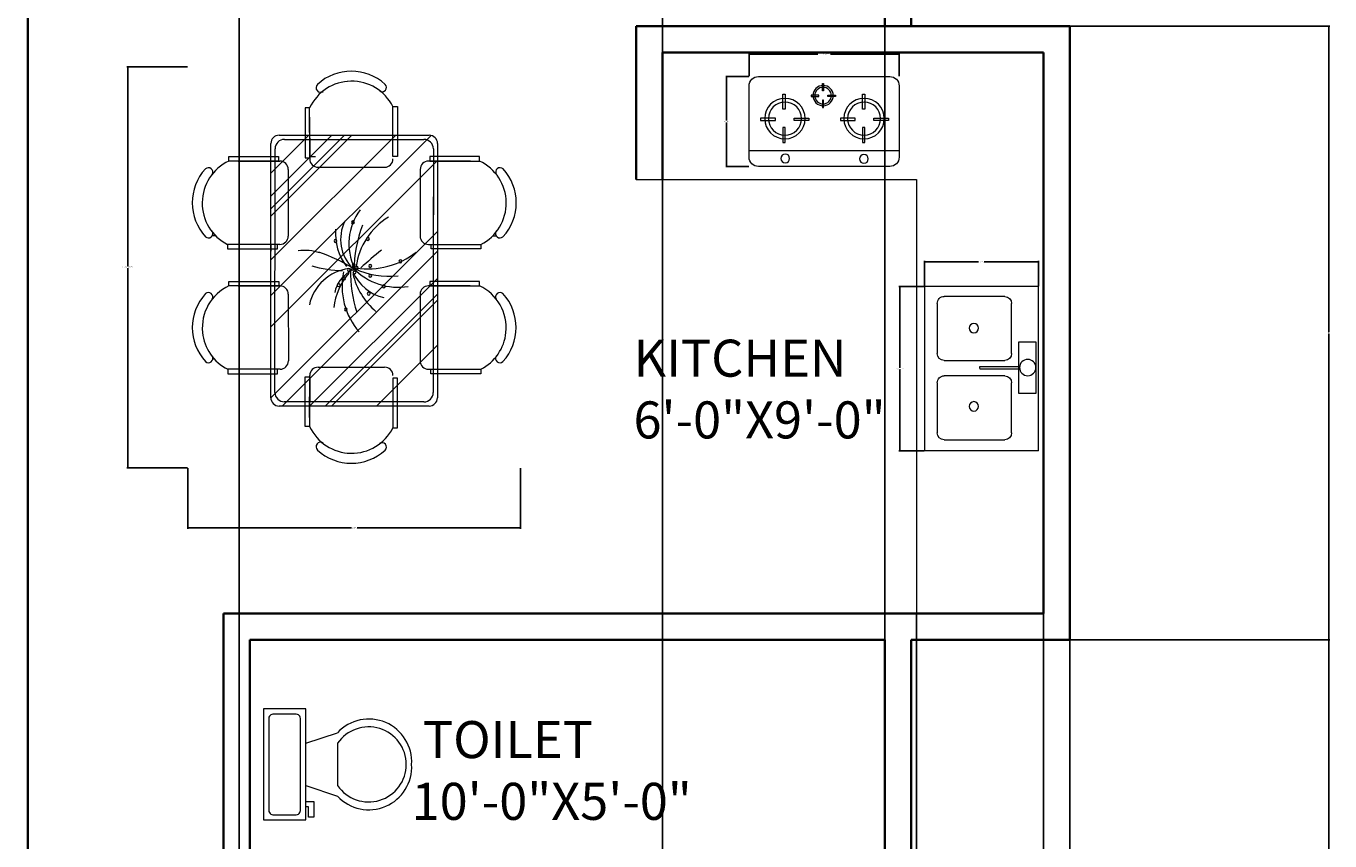
# Model space of a CAD drawing. Units: inches. Extents: x 3731 to 4318, y 1310 to 2388.
# Tile 31 of 57: x 4072 to 4318, y 1554 to 1708. Entities that reach past the tile are written whole.
import ezdxf

# ---------------------------------------------------------------- set-up
doc = ezdxf.new("R2010")
doc.units = ezdxf.units.IN
for name, color, linetype, lineweight in [('A-ANNO-DIMS', 2, 'Continuous', 18), ('A-AREA-IDEN', 7, 'Continuous', 18), ('A-EQPM', 8, 'Continuous', 18), ('A-FLOR-CASE', 8, 'Continuous', 18), ('A-FLOR-FIXT', 9, 'Continuous', 18), ('A-FURN', 8, 'Continuous', 13), ('A-WALL', 7, 'Continuous', 35)]:
    doc.layers.add(name, color=color, linetype=linetype, lineweight=lineweight)
doc.styles.get("Standard").update_dxf_attribs({"font": 'arial.ttf'})
doc.dimstyles.get("Standard").update_dxf_attribs({"dimtxt": 0.18, "dimasz": 0.18, "dimexe": 0.18, "dimexo": 0.0625, "dimgap": 0.09, "dimtad": 0, "dimtih": 1, "dimtoh": 1, "dimdec": 4, "dimzin": 0, "dimdsep": 46, "dimtxsty": 'Standard', "dimcen": 0.09, "dimadec": 0, "dimazin": 0, "dimtfac": 1, "dimtdec": 4, "dimtofl": 0, "dimtmove": 0, "dimatfit": 3, "dimfxl": 1, "dimtolj": 1, "dimtzin": 0, "dimarcsym": 0})

# ---------------------------------------------------------------- blocks, each defined once
blk = doc.blocks.new('A$C6327331B')
for p, q in [((790.8, 678.3), (790.8, 696.4)), ((790.8, 678.3), (790.8, 696.4)), ((1381.3, 692.8), (1381.3, 686.2)), ((1381.3, 692.8), (1381.3, 686.2)), ((410.1, 615.8), (410, 377)), ((410.1, 615.8), (410, 377)), ((431.6, 615.8), (410.1, 615.8)), ((431.6, 615.8), (410.1, 615.8)), ((431.4, 376.9), (431.6, 615.8)), ((431.4, 376.9), (431.6, 615.8)), ((431.5, 571.8), (431.4, 370.8)), ((431.5, 571.8), (431.4, 370.8)), ((831.4, 382.9), (831.6, 621.7)), ((831.4, 382.9), (831.6, 621.7)), ((831.4, 370.6), (831.5, 571.6)), ((831.4, 370.6), (831.5, 571.6)), ((831.6, 621.7), (853, 621.7)), ((831.6, 621.7), (853, 621.7)), ((853, 621.7), (852.9, 382.9)), ((853, 621.7), (852.9, 382.9)), ((1009.3, 615.5), (1009.2, 376.7)), ((1009.3, 615.5), (1009.2, 376.7)), ((1030.7, 615.5), (1009.3, 615.5)), ((1030.7, 615.5), (1009.3, 615.5)), ((1030.6, 376.6), (1030.7, 615.5)), ((1030.6, 376.6), (1030.7, 615.5)), ((1030.7, 571.5), (1030.6, 370.5)), ((1030.7, 571.5), (1030.6, 370.5)), ((1430.6, 382.6), (1430.7, 621.4)), ((1430.6, 382.6), (1430.7, 621.4)), ((1430.6, 370.3), (1430.7, 571.3)), ((1430.6, 370.3), (1430.7, 571.3)), ((1430.7, 621.4), (1452.2, 621.4)), ((1430.7, 621.4), (1452.2, 621.4)), ((1452.2, 621.4), (1452, 382.6)), ((1452.2, 621.4), (1452, 382.6)), ((1075.9, -386.3), (308.5, 383.1)), ((1075.9, -386.3), (308.5, 383.1)), ((347.5, 414), (831.5, 413.8)), ((347.5, 414), (831.5, 413.8)), ((372.5, 394), (831.4, 393.8)), ((372.5, 394), (1009.2, 393.7)), ((410, 377), (431.4, 376.9)), ((410, 377), (431.4, 376.9)), ((1226.3, -386.4), (428, 414)), ((1226.3, -386.4), (428, 414)), ((1567.1, -386.6), (768.8, 413.8)), ((1567.1, -386.6), (768.8, 413.8)), ((852.9, 382.9), (831.4, 382.9)), ((852.9, 382.9), (831.4, 382.9)), ((831.5, 413.8), (1567.5, 413.4)), ((1607.1, -331.3), (864.1, 413.8)), ((1607.1, -331.3), (864.1, 413.8)), ((1607.2, -200.8), (994.4, 413.7)), ((1607.2, -200.8), (994.4, 413.7)), ((1009.2, 413.7), (1567.5, 413.4)), ((1009.2, 393.7), (1542.5, 393.4)), ((1009.2, 376.7), (1030.6, 376.6)), ((1009.2, 376.7), (1030.6, 376.6)), ((1607.2, -125.5), (1069.5, 413.7)), ((1607.2, -125.5), (1069.5, 413.7)), ((1607.2, -95.4), (1099.6, 413.6)), ((1607.2, -95.4), (1099.6, 413.6)), ((1607.3, 120.5), (1315.1, 413.5)), ((1607.3, 120.5), (1315.1, 413.5)), ((1415.7, 413.4), (1415.7, 413.5)), ((1415.7, 413.4), (1415.7, 413.5)), ((1452, 382.6), (1430.6, 382.6)), ((1452, 382.6), (1430.6, 382.6)), ((307.1, -346), (307.5, 374)), ((307.1, -346), (307.5, 374)), ((327.1, -321), (327.5, 349)), ((471.4, 330.8), (791.4, 330.6)), ((471.4, 330.8), (791.4, 330.6)), ((1070.6, 330.5), (1390.6, 330.3)), ((1070.6, 330.5), (1390.6, 330.3)), ((1587.5, 348.4), (1587.1, -321.6)), ((1607.5, 373.4), (1607.1, -346.6)), ((1607.5, 373.4), (1607.1, -346.6)), ((169.9, 221.5), (408.7, 221.6)), ((169.9, 221.5), (408.7, 221.6)), ((169.9, 200.1), (169.9, 221.5)), ((169.9, 200.1), (169.9, 221.5)), ((408.7, 200.2), (169.9, 200.1)), ((408.7, 200.2), (169.9, 200.1)), ((905.5, -386.3), (307.4, 213.5)), ((905.5, -386.3), (307.4, 213.5)), ((408.7, 221.6), (408.7, 200.2)), ((408.7, 221.6), (408.7, 200.2)), ((1473.3, 221.6), (1473.3, 200.2)), ((1473.3, 221.6), (1473.3, 200.2)), ((1712.1, 221.5), (1473.3, 221.6)), ((1712.1, 221.5), (1473.3, 221.6)), ((1473.3, 200.2), (1712.1, 200.1)), ((1473.3, 200.2), (1712.1, 200.1)), ((1712.1, 200.1), (1712.1, 221.5)), ((1712.1, 200.1), (1712.1, 221.5)), ((461.2, -159.8), (461, 160.2)), ((461.2, -159.8), (461, 160.2)), ((1420.8, -159.8), (1420.9, 160.2)), ((1420.8, -159.8), (1420.9, 160.2)), ((695.1, -386.2), (307.3, 2.7)), ((695.1, -386.2), (307.3, 2.7)), ((44.6, -20.2), (44.5, -20.1)), ((44.6, -20.2), (44.5, -20.1)), ((660, -386.1), (307.3, -32.5)), ((660, -386.1), (307.3, -32.5)), ((1837.4, -20.2), (1837.5, -20.1)), ((1837.4, -20.2), (1837.5, -20.1)), ((599.8, -386.1), (307.2, -92.7)), ((599.8, -386.1), (307.2, -92.7)), ((408.7, -193.6), (408.7, -172.1)), ((408.7, -193.6), (408.7, -172.1)), ((415.1, -199.8), (176.2, -199.9)), ((415.1, -199.8), (176.2, -199.9)), ((176.2, -199.9), (176.2, -221.3)), ((176.2, -199.9), (176.2, -221.3)), ((176.2, -221.3), (415.1, -221.2)), ((176.2, -221.3), (415.1, -221.2)), ((220.2, -199.9), (421.2, -199.8)), ((220.2, -199.9), (421.2, -199.8)), ((489.6, -386), (307.2, -203.2)), ((489.6, -386), (307.2, -203.2)), ((415.1, -221.2), (415.1, -199.8)), ((415.1, -221.2), (415.1, -199.8)), ((1661.8, -199.9), (1460.8, -199.8)), ((1661.8, -199.9), (1460.8, -199.8)), ((1466.9, -221.2), (1466.9, -199.8)), ((1466.9, -221.2), (1466.9, -199.8)), ((1466.9, -199.8), (1705.7, -199.9)), ((1466.9, -199.8), (1705.7, -199.9)), ((1705.7, -221.3), (1466.9, -221.2)), ((1705.7, -221.3), (1466.9, -221.2)), ((1705.7, -199.9), (1705.7, -221.3)), ((1705.7, -199.9), (1705.7, -221.3)), ((471.4, -302.7), (791.4, -302.5)), ((471.4, -302.7), (791.4, -302.5)), ((1070.6, -302.4), (1390.6, -302.2)), ((1070.6, -302.4), (1390.6, -302.2)), ((1542.1, -366.6), (372.1, -366)), ((410.1, -587.7), (410, -348.9)), ((410.1, -587.7), (410, -348.9)), ((410, -348.9), (431.4, -348.9)), ((410, -348.9), (431.4, -348.9)), ((431.5, -543.7), (431.4, -342.7)), ((431.5, -543.7), (431.4, -342.7)), ((431.4, -348.9), (431.6, -587.7)), ((431.4, -348.9), (431.6, -587.7)), ((831.4, -342.5), (831.5, -543.5)), ((831.4, -342.5), (831.5, -543.5)), ((831.4, -354.8), (831.6, -593.6)), ((831.4, -354.8), (831.6, -593.6)), ((852.9, -354.8), (831.4, -354.8)), ((852.9, -354.8), (831.4, -354.8)), ((853, -593.6), (852.9, -354.8)), ((853, -593.6), (852.9, -354.8)), ((1009.2, -348.6), (1030.6, -348.5)), ((1009.2, -348.6), (1030.6, -348.5)), ((1009.3, -587.4), (1009.2, -348.6)), ((1009.3, -587.4), (1009.2, -348.6)), ((1030.7, -543.4), (1030.6, -342.4)), ((1030.7, -543.4), (1030.6, -342.4)), ((1030.6, -348.5), (1030.7, -587.4)), ((1030.6, -348.5), (1030.7, -587.4)), ((1430.6, -342.2), (1430.7, -543.2)), ((1430.6, -342.2), (1430.7, -543.2)), ((1430.6, -354.5), (1430.7, -593.3)), ((1430.6, -354.5), (1430.7, -593.3)), ((1452, -354.5), (1430.6, -354.5)), ((1452, -354.5), (1430.6, -354.5)), ((1452.2, -593.3), (1452, -354.5)), ((1452.2, -593.3), (1452, -354.5)), ((1567.1, -386.6), (347.1, -386)), ((1567.1, -386.6), (347.1, -386)), ((831.5, -385.7), (864.1, -385.7)), ((831.5, -385.7), (864.1, -385.7)), ((1415.7, -385.3), (1415.7, -385.4)), ((1415.7, -385.3), (1415.7, -385.4)), ((431.6, -587.7), (410.1, -587.7)), ((431.6, -587.7), (410.1, -587.7)), ((831.6, -593.6), (853, -593.6)), ((831.6, -593.6), (853, -593.6)), ((1030.7, -587.4), (1009.3, -587.4)), ((1030.7, -587.4), (1009.3, -587.4)), ((1430.7, -593.3), (1452.2, -593.3)), ((1430.7, -593.3), (1452.2, -593.3)), ((790.8, -650.2), (790.8, -668.4)), ((790.8, -650.2), (790.8, -668.4)), ((1381.3, -664.7), (1381.3, -658.1)), ((1381.3, -664.7), (1381.3, -658.1))]:
    blk.add_line(p, q)
for centre, radius, start, end in [((631.5, 550.5), 241.3, 47.46915, 132.47205), ((631.5, 550.5), 241.3, 47.46915, 132.47205), ((1230.7, 550.2), 241.3, 47.46915, 132.47205), ((1230.7, 550.2), 241.3, 47.46915, 132.47205), ((633, 521.6), 222.4, 26.76564, 154.93691), ((633, 521.6), 222.4, 26.76564, 154.93691), ((484.3, 714.2), 21.2, 137.64965, 300.34124), ((484.3, 714.2), 21.2, 137.64965, 300.34124), ((779, 714), 21.2, 239.59996, 42.29154), ((779, 714), 21.2, 239.59996, 42.29154), ((1232.2, 521.3), 222.4, 84.42654, 154.93691), ((1232.2, 521.3), 222.4, 84.42654, 154.93691), ((1083.4, 713.9), 21.2, 137.64965, 300.34124), ((1083.4, 713.9), 21.2, 137.64965, 300.34124), ((1232.2, 521.3), 222.4, 26.76564, 84.42654), ((1232.2, 521.3), 222.4, 26.76564, 84.42654), ((1378.1, 713.7), 21.2, 239.59996, 42.29154), ((1378.1, 713.7), 21.2, 239.59996, 42.29154), ((347.5, 374), 40, 89.9706, 179.9706), ((347.5, 374), 40, 89.9706, 179.9706), ((372.5, 349), 45, 89.9706, 179.9706), ((1542.5, 348.4), 45, 359.9706, 89.9706), ((1567.5, 373.4), 40, 359.9706, 89.9706), ((1567.5, 373.4), 40, 359.9706, 89.9706), ((471.4, 370.8), 40, 179.9706, 269.9706), ((471.4, 370.8), 40, 179.9706, 269.9706), ((791.4, 370.6), 40, 269.9706, 359.9706), ((791.4, 370.6), 40, 269.9706, 359.9706), ((1070.6, 370.5), 40, 179.9706, 269.9706), ((1070.6, 370.5), 40, 179.9706, 269.9706), ((1390.6, 370.3), 40, 269.9706, 359.9706), ((1390.6, 370.3), 40, 269.9706, 359.9706), ((574.1, 79.9), 374.6, 351.24958, 38.23328), ((737.8, 225), 299.2, 314.48606, 9.37622), ((270.2, 1.6), 222.4, 116.82445, 244.99571), ((270.2, 1.6), 222.4, 116.82445, 244.99571), ((421, 160.2), 40, 0.0294, 90.0294), ((421, 160.2), 40, 0.0294, 90.0294), ((912.6, 235.7), 6.91, 0, 180), ((912.6, 235.7), 6.91, 180, 0), ((586.4, 182.9), 398.1, 335.08876, 5.96372), ((1460.9, 160.2), 40, 89.9706, 179.9706), ((1460.9, 160.2), 40, 89.9706, 179.9706), ((1611.7, 1.6), 222.4, 295.00429, 63.17555), ((1611.7, 1.6), 222.4, 295.00429, 63.17555), ((241.3, 0.1), 241.3, 137.52795, 222.53085), ((77.6, 147.4), 21.2, 329.65876, 132.35035), ((77.6, 147.4), 21.2, 329.65876, 132.35035), ((983.2, 350.8), 331, 211.31505, 262.13779), ((2460.3, 1443.6), 2062.1, 219.04877, 222.6799), ((873.8, 207.8), 219.3, 294.09558, 346.29534), ((1033, 155.9), 6.91, 0, 180), ((1033, 155.9), 6.91, 180, 0), ((1804.4, 147.4), 21.2, 47.64965, 210.34124), ((1804.4, 147.4), 21.2, 47.64965, 210.34124), ((1640.7, 0.1), 241.3, 317.46915, 42.47205), ((1640.7, 0.1), 241.3, 317.46915, 42.47205), ((805, 79.9), 6.91, 0, 180), ((805, 79.9), 6.91, 180, 0), ((934.8, 91.3), 6.91, 0, 180), ((934.8, 91.3), 6.91, 180, 0), ((897.1, 334.6), 335.6, 283.04524, 319.77663), ((982.3, 91.3), 6.91, 0, 180), ((982.3, 91.3), 6.91, 180, 0), ((1067.8, 83.7), 6.91, 0, 180), ((1067.8, 83.7), 6.91, 180, 0), ((826.9, 258.5), 270.1, 233.32313, 295.76326), ((725.8, 7.7), 6.91, 0, 180), ((725.8, 7.7), 6.91, 180, 0), ((807.8, 143), 194.5, 242.99086, 315.91017), ((985.1, 750.7), 739.8, 250.5249, 267.82437), ((1747.6, -469.5), 933.6, 148.98728, 160.36101), ((931.7, 11.5), 6.91, 0, 180), ((931.7, 11.5), 6.91, 180, 0), ((944.3, 26.7), 6.91, 0, 180), ((944.3, 26.7), 6.91, 180, 0), ((947.5, 3.9), 6.91, 0, 180), ((947.5, 3.9), 6.91, 180, 0), ((970.7, 574.8), 578.8, 268.32856, 288.729), ((966.5, 15.3), 6.91, 0, 180), ((966.5, 15.3), 6.91, 180, 0), ((1030.3, 292.7), 337.4, 258.55155, 310.98153), ((776.7, 191.6), 268.2, 265.87406, 306.95584), ((392.7, -33), 564.4, 343.85612, 359.11051), ((953.8, -11.3), 6.91, 0, 180), ((953.8, -11.3), 6.91, 180, 0), ((1167.7, 15.7), 221.9, 186.99045, 258.02836), ((1090.6, 62.7), 145.4, 208.89012, 258.45792), ((1166.2, 212.9), 298.2, 228.7581, 263.8624), ((995, -34.1), 6.91, 0, 180), ((995, -34.1), 6.91, 180, 0), ((1026.7, -60.7), 6.91, 0, 180), ((1026.7, -60.7), 6.91, 180, 0), ((1143.8, -26.5), 6.91, 0, 180), ((1143.8, -26.5), 6.91, 180, 0), ((814.5, -75.9), 6.91, 0, 180), ((814.5, -75.9), 6.91, 180, 0), ((79, -146.7), 22.5, 226.37763, 29.88821), ((79, -146.7), 22.5, 226.37763, 29.88821), ((421.2, -159.8), 40, 270.0294, 0.0294), ((421.2, -159.8), 40, 270.0294, 0.0294), ((1112.9, -226), 252.6, 162.94564, 186.48138), ((1460.8, -159.8), 40, 179.9706, 269.9706), ((1460.8, -159.8), 40, 179.9706, 269.9706), ((1803, -146.7), 22.5, 150.11179, 313.62237), ((1803, -146.7), 22.5, 150.11179, 313.62237), ((471.4, -342.7), 40, 90.0294, 180.0294), ((471.4, -342.7), 40, 90.0294, 180.0294), ((791.4, -342.5), 40, 0.0294, 90.0294), ((791.4, -342.5), 40, 0.0294, 90.0294), ((1070.6, -342.4), 40, 90.0294, 180.0294), ((1070.6, -342.4), 40, 90.0294, 180.0294), ((1390.6, -342.2), 40, 0.0294, 90.0294), ((1390.6, -342.2), 40, 0.0294, 90.0294), ((347.1, -346), 40, 179.9706, 269.9706), ((347.1, -346), 40, 179.9706, 269.9706), ((372.1, -321), 45, 179.9706, 269.9706), ((1542.1, -321.6), 45, 269.9706, 359.9706), ((1567.1, -346.6), 40, 269.9706, 359.9706), ((1567.1, -346.6), 40, 269.9706, 359.9706), ((633, -493.5), 222.4, 205.06309, 333.23436), ((633, -493.5), 222.4, 205.06309, 333.23436), ((1232.2, -493.2), 222.4, 205.06309, 275.57346), ((1232.2, -493.2), 222.4, 205.06309, 275.57346), ((1232.2, -493.2), 222.4, 275.57346, 333.23436), ((1232.2, -493.2), 222.4, 275.57346, 333.23436), ((484.3, -686.1), 21.2, 59.65876, 222.35035), ((484.3, -686.1), 21.2, 59.65876, 222.35035), ((779, -686), 21.2, 317.70846, 120.40004), ((779, -686), 21.2, 317.70846, 120.40004), ((1083.4, -685.8), 21.2, 59.65876, 222.35035), ((1083.4, -685.8), 21.2, 59.65876, 222.35035), ((1378.1, -685.6), 21.2, 317.70846, 120.40004), ((1378.1, -685.6), 21.2, 317.70846, 120.40004), ((631.5, -522.4), 241.3, 227.52795, 312.53085), ((631.5, -522.4), 241.3, 227.52795, 312.53085), ((1230.7, -522.1), 241.3, 227.52795, 312.53085), ((1230.7, -522.1), 241.3, 227.52795, 312.53085)]:
    blk.add_arc(centre, radius, start, end)
at = {"width": 0.8, "flags": 9}
for tag in ['XSIZE', 'YSIZE']:
    blk.add_attdef(tag, (945.2, 11.4), '', height=0.23, rotation=180, dxfattribs=at)
blk = doc.blocks.new('*U14')
for p, q in [((9.5, -6), (9.5, -2)), ((-10, -8.5), (-8, -8.5)), ((-10, -9.5), (-10, -8.5)), ((-7, -9.5), (-10, -9.5)), ((-8, -8.5), (-8, -8)), ((-7, -8), (-7, -9.5)), ((-4, -8), (-6, -14)), ((4, -8), (6, -14)), ((4, -14), (-4, -14))]:
    blk.add_line(p, q)
blk.add_lwpolyline([(10.5, -8), (10.5, 0), (-10.5, 0), (-10.5, -8)], close=True)
for points in [[(-9.5, -2), (-9.5, -6)], [(8.5, -1), (-8.5, -1)], [(-8.5, -7), (8.5, -7)]]:
    blk.add_lwpolyline(points)
for centre, radius, start, end in [((-8.625, -1.875), 0.8839, 81.8699, 188.1301), ((8.625, -1.875), 0.8839, 351.8699, 98.1301), ((-8.625, -6.125), 0.8839, 171.869898, 278.1301), ((8.625, -6.125), 0.8839, 261.8699, 8.1301), ((-0.4772, -19.9188), 8.0953, 133.01722, 273.38), ((0.0374, -19.8731), 7.127, 124.50543, 269.7), ((-0.0373, -19.8731), 7.127, 270.3, 55.4946), ((0.4773, -19.9188), 8.0953, 266.62, 46.9828)]:
    blk.add_arc(centre, radius, start, end)
blk = doc.blocks.new('A$C2A3C6842')
for p, q in [((0, 45), (0, 387)), ((45, 432), (675, 432)), ((351.6, 363.3), (351.6, 398.9)), ((351.6, 398.9), (357.3, 398.9)), ((357.3, 398.9), (357.3, 363.3)), ((720, 387), (720, 45)), ((161.8, 346.9), (173.2, 346.9)), ((161.8, 275.6), (161.8, 346.9)), ((173.2, 346.9), (173.2, 275.6)), ((298.4, 341.9), (298.4, 336.2)), ((334, 341.9), (298.4, 341.9)), ((298.4, 336.2), (334, 336.2)), ((334, 336.2), (334, 341.9)), ((357.3, 363.3), (351.6, 363.3)), ((357.3, 318.8), (351.6, 318.8)), ((351.6, 318.8), (351.6, 283.1)), ((357.3, 283.1), (357.3, 318.8)), ((378.5, 336.2), (378.5, 341.9)), ((378.5, 341.9), (414.2, 341.9)), ((414.2, 336.2), (378.5, 336.2)), ((414.2, 341.9), (414.2, 336.2)), ((544.7, 346.9), (556.1, 346.9)), ((544.7, 275.6), (544.7, 346.9)), ((556.1, 346.9), (556.1, 275.6)), ((173.2, 275.6), (161.8, 275.6)), ((351.6, 283.1), (357.3, 283.1)), ((556.1, 275.6), (544.7, 275.6)), ((55.3, 232.9), (55.3, 221.5)), ((126.6, 232.9), (55.3, 232.9)), ((55.3, 221.5), (126.6, 221.5)), ((126.6, 221.5), (126.6, 232.9)), ((215.6, 221.5), (215.6, 232.9)), ((215.6, 232.9), (286.9, 232.9)), ((286.9, 221.5), (215.6, 221.5)), ((286.9, 232.9), (286.9, 221.5)), ((438.2, 232.9), (438.2, 221.5)), ((509.5, 232.9), (438.2, 232.9)), ((438.2, 221.5), (509.5, 221.5)), ((509.5, 221.5), (509.5, 232.9)), ((598.5, 232.9), (669.8, 232.9)), ((598.5, 221.5), (598.5, 232.9)), ((669.8, 221.5), (598.5, 221.5)), ((669.8, 232.9), (669.8, 221.5)), ((173.2, 186.6), (161.8, 186.6)), ((161.8, 186.6), (161.8, 115.3)), ((173.2, 115.3), (173.2, 186.6)), ((556.1, 186.6), (544.7, 186.6)), ((544.7, 186.6), (544.7, 115.3)), ((556.1, 115.3), (556.1, 186.6)), ((1.2, 76.7), (719.9, 76.7)), ((161.8, 115.3), (173.2, 115.3)), ((544.7, 115.3), (556.1, 115.3)), ((675, 0), (45, 0))]:
    blk.add_line(p, q)
at = {"extrusion": (0, -1e-16, -1)}
for centre, major_axis, start_param, end_param in [((45, 387), (31.8, 31.8), 3.926991, 5.497787), ((172.2, 229.8), (-97.3, 0.1), -0.001099, 6.282086), ((551.8, 229.8), (-97.3, 0.1), -0.001099, 6.282086), ((173.7, 39), (-14.8, 14.8), 5.497787, 11.780972)]:
    blk.add_ellipse(centre, major_axis=major_axis, ratio=1, start_param=start_param, end_param=end_param, dxfattribs=at)
at = {"extrusion": (-1e-16, -1e-16, -1)}
blk.add_ellipse((355.1, 340.4), major_axis=(48.7, 0.1), ratio=1, start_param=3.144125, end_param=9.42731, dxfattribs=at)
at = {"extrusion": (-1e-16, 0, -1)}
for centre, major_axis, start_param, end_param in [((355.1, 340.4), (-39.7, 0), -0.000334, 6.282851), ((45, 45), (-31.8, 31.8), 3.926991, 5.497787)]:
    blk.add_ellipse(centre, major_axis=major_axis, ratio=1, start_param=start_param, end_param=end_param, dxfattribs=at)
at = {"extrusion": (0, 1e-16, -1)}
blk.add_ellipse((675, 387), major_axis=(-31.8, 31.8), ratio=1, start_param=0.785398, end_param=2.356194, dxfattribs=at)
at = {"extrusion": (-1e-16, -4e-16, -1)}
for centre in [(172.2, 229.8), (551.8, 229.8)]:
    blk.add_ellipse(centre, major_axis=(-79.3, 0), ratio=1, start_param=-0.0002116186602152, end_param=6.282973688519371, dxfattribs=at)
at = {"extrusion": (2e-16, -2e-16, -1)}
blk.add_ellipse((551.4, 36.4), major_axis=(14.8, 14.8), ratio=1, start_param=3.926991, end_param=10.210176, dxfattribs=at)
at = {"extrusion": (-2e-16, 1e-16, -1)}
blk.add_ellipse((675, 45), major_axis=(31.8, 31.8), ratio=1, start_param=0.785398, end_param=2.356194, dxfattribs=at)
at = {"text_generation_flag": 4, "flags": 9}
for tag in ['XSIZE', 'YSIZE']:
    blk.add_attdef(tag, (361.3, 264.9), '', height=0.45, rotation=180, dxfattribs=at)
blk = doc.blocks.new('A$C3AD04490')
for p, q in [((0, 640.7), (0, 0)), ((0, 640.7), (924.9, 640.7)), ((614, 627.3), (322.5, 627.3)), ((322.5, 627.3), (322.5, 531.5)), ((614, 531.5), (614, 627.3)), ((924.9, 640.7), (924.9, 0)), ((322.5, 531.5), (614, 531.5)), ((462.6, 311.9), (462.6, 537.2)), ((473.8, 536.8), (473.8, 311.9)), ((62.3, 110.9), (62.3, 451.4)), ((101.4, 490.5), (383.1, 490.5)), ((422.3, 451.4), (422.3, 110.9)), ((508.8, 110.9), (508.8, 451.4)), ((547.9, 490.5), (829.6, 490.5)), ((868.8, 451.4), (868.8, 110.9)), ((463.4, 310.9), (474.3, 310.9)), ((383.1, 71.7), (101.4, 71.7)), ((829.6, 71.7), (547.9, 71.7)), ((924.9, 0), (0, 0))]:
    blk.add_line(p, q)
for centre, radius in [((469, 581.2), 45.9), ((250.7, 278.1), 26.4), ((690.5, 278.1), 26.4)]:
    blk.add_circle(centre, radius)
for centre, start, end in [((101.4, 451.4), 90, 180), ((383.1, 451.4), 0, 90), ((547.9, 451.4), 90, 180), ((829.6, 451.4), 0, 90), ((101.4, 110.9), 180, 270), ((383.1, 110.9), 270, 0), ((547.9, 110.9), 180, 270), ((829.6, 110.9), 270, 0)]:
    blk.add_arc(centre, 39.1, start, end)
blk = doc.blocks.new('*D24')
at = {"layer": 'A-ANNO-DIMS', "color": 0, "lineweight": -2, "transparency": 16777216}
for p, q in [((4102.42, 1700.68), (4090.94, 1700.68)), ((4091.12, 1700.5), (4091.12, 1662.99)), ((4091.12, 1625.1), (4091.12, 1662.62)), ((4102.42, 1624.92), (4090.94, 1624.92))]:
    blk.add_line(p, q, dxfattribs=at)
at = {"layer": 'A-ANNO-DIMS', "color": 0, "transparency": 16777216}
for points in [[(4091.09, 1700.5), (4091.15, 1700.5), (4091.12, 1700.68)], [(4091.09, 1625.1), (4091.15, 1625.1), (4091.12, 1624.92)]]:
    blk.add_solid(points, dxfattribs=at)
at = {"layer": 'Defpoints', "color": 0, "transparency": 16777216}
for p in [(4102.48, 1700.68), (4091.12, 1624.92), (4102.48, 1624.92)]:
    blk.add_point(p, dxfattribs=at)
at = {"layer": 'A-ANNO-DIMS', "color": 0, "transparency": 16777216, "insert": (4091.12, 1662.8), "char_height": 0.18, "attachment_point": 5}
blk.add_mtext('\\A1;DINING SET 76 TYP.', dxfattribs=at)
blk = doc.blocks.new('*D25')
at = {"layer": 'A-ANNO-DIMS', "color": 0, "lineweight": -2, "transparency": 16777216}
for p, q in [((4102.48, 1624.86), (4102.48, 1613.38)), ((4165.39, 1624.86), (4165.39, 1613.38)), ((4102.66, 1613.56), (4133.41, 1613.56)), ((4165.21, 1613.56), (4134.46, 1613.56))]:
    blk.add_line(p, q, dxfattribs=at)
at = {"layer": 'A-ANNO-DIMS', "color": 0, "transparency": 16777216}
for points in [[(4102.66, 1613.59), (4102.66, 1613.53), (4102.48, 1613.56)], [(4165.21, 1613.59), (4165.21, 1613.53), (4165.39, 1613.56)]]:
    blk.add_solid(points, dxfattribs=at)
at = {"layer": 'Defpoints', "color": 0, "transparency": 16777216}
for p in [(4102.48, 1624.92), (4165.39, 1624.92), (4165.39, 1613.56)]:
    blk.add_point(p, dxfattribs=at)
at = {"layer": 'A-ANNO-DIMS', "color": 0, "transparency": 16777216, "insert": (4133.93, 1613.56), "char_height": 0.18, "attachment_point": 5}
blk.add_mtext('\\A1;63 TYP.', dxfattribs=at)
blk = doc.blocks.new('*D26')
at = {"layer": 'A-ANNO-DIMS', "color": 0, "lineweight": -2, "transparency": 16777216}
for p, q in [((4241.66, 1659.17), (4236.88, 1659.17)), ((4237.06, 1658.99), (4237.06, 1643.82)), ((4237.06, 1628.27), (4237.06, 1643.45)), ((4241.66, 1628.09), (4236.88, 1628.09))]:
    blk.add_line(p, q, dxfattribs=at)
at = {"layer": 'A-ANNO-DIMS', "color": 0, "transparency": 16777216}
for points in [[(4237.03, 1658.99), (4237.09, 1658.99), (4237.06, 1659.17)], [(4237.03, 1628.27), (4237.09, 1628.27), (4237.06, 1628.09)]]:
    blk.add_solid(points, dxfattribs=at)
at = {"layer": 'Defpoints', "color": 0, "transparency": 16777216}
for p in [(4237.06, 1659.17), (4241.72, 1659.17), (4241.72, 1628.09)]:
    blk.add_point(p, dxfattribs=at)
at = {"layer": 'A-ANNO-DIMS', "color": 0, "transparency": 16777216, "insert": (4237.06, 1643.63), "char_height": 0.18, "attachment_point": 5}
blk.add_mtext('\\A1;SINK 31 TYP.', dxfattribs=at)
blk = doc.blocks.new('*D27')
at = {"layer": 'A-ANNO-DIMS', "color": 0, "lineweight": -2, "transparency": 16777216}
for p, q in [((4241.72, 1659.23), (4241.72, 1664.01)), ((4241.9, 1663.83), (4251.96, 1663.83)), ((4263.07, 1663.83), (4253.02, 1663.83)), ((4263.25, 1659.23), (4263.25, 1664.01))]:
    blk.add_line(p, q, dxfattribs=at)
at = {"layer": 'A-ANNO-DIMS', "color": 0, "transparency": 16777216}
for points in [[(4241.9, 1663.86), (4241.9, 1663.8), (4241.72, 1663.83)], [(4263.07, 1663.86), (4263.07, 1663.8), (4263.25, 1663.83)]]:
    blk.add_solid(points, dxfattribs=at)
at = {"layer": 'Defpoints', "color": 0, "transparency": 16777216}
for p in [(4263.25, 1663.83), (4241.72, 1659.17), (4263.25, 1659.17)]:
    blk.add_point(p, dxfattribs=at)
at = {"layer": 'A-ANNO-DIMS', "color": 0, "transparency": 16777216, "insert": (4252.49, 1663.83), "char_height": 0.18, "attachment_point": 5}
blk.add_mtext('\\A1;22 TYP.', dxfattribs=at)
blk = doc.blocks.new('*D28')
at = {"layer": 'A-ANNO-DIMS', "color": 0, "lineweight": -2, "transparency": 16777216}
for p, q in [((4208.58, 1698.91), (4208.58, 1703.28)), ((4208.76, 1703.1), (4221.57, 1703.1)), ((4236.75, 1703.1), (4223.95, 1703.1)), ((4236.93, 1698.91), (4236.93, 1703.28))]:
    blk.add_line(p, q, dxfattribs=at)
at = {"layer": 'A-ANNO-DIMS', "color": 0, "transparency": 16777216}
for points in [[(4208.76, 1703.13), (4208.76, 1703.07), (4208.58, 1703.1)], [(4236.75, 1703.13), (4236.75, 1703.07), (4236.93, 1703.1)]]:
    blk.add_solid(points, dxfattribs=at)
at = {"layer": 'Defpoints', "color": 0, "transparency": 16777216}
for p in [(4236.93, 1703.1), (4208.58, 1698.85), (4236.93, 1698.85)]:
    blk.add_point(p, dxfattribs=at)
at = {"layer": 'A-ANNO-DIMS', "color": 0, "transparency": 16777216, "insert": (4222.76, 1703.1), "char_height": 0.18, "attachment_point": 5}
blk.add_mtext('\\A1;COOKTOP 28 TYP.', dxfattribs=at)
blk = doc.blocks.new('*D29')
at = {"layer": 'A-ANNO-DIMS', "color": 0, "lineweight": -2, "transparency": 16777216}
for p, q in [((4208.52, 1698.85), (4204.15, 1698.85)), ((4204.33, 1698.67), (4204.33, 1690.53)), ((4204.33, 1682.02), (4204.33, 1690.17)), ((4208.52, 1681.84), (4204.15, 1681.84))]:
    blk.add_line(p, q, dxfattribs=at)
at = {"layer": 'A-ANNO-DIMS', "color": 0, "transparency": 16777216}
for points in [[(4204.3, 1698.67), (4204.36, 1698.67), (4204.33, 1698.85)], [(4204.3, 1682.02), (4204.36, 1682.02), (4204.33, 1681.84)]]:
    blk.add_solid(points, dxfattribs=at)
at = {"layer": 'Defpoints', "color": 0, "transparency": 16777216}
for p in [(4204.33, 1698.85), (4208.58, 1698.85), (4208.58, 1681.84)]:
    blk.add_point(p, dxfattribs=at)
at = {"layer": 'A-ANNO-DIMS', "color": 0, "transparency": 16777216, "insert": (4204.33, 1690.35), "char_height": 0.18, "attachment_point": 5}
blk.add_mtext('\\A1;17 TYP.', dxfattribs=at)
blk = doc.blocks.new('*D32')
at = {"layer": 'A-ANNO-DIMS', "color": 0, "lineweight": -2, "transparency": 16777216}
for p, q in [((4269.21, 1592.32), (4269.21, 1310.25)), ((3835.21, 1359.32), (3835.21, 1310.25)), ((3835.39, 1310.43), (4051.92, 1310.43)), ((4269.03, 1310.43), (4052.5, 1310.43))]:
    blk.add_line(p, q, dxfattribs=at)
at = {"layer": 'A-ANNO-DIMS', "color": 0, "transparency": 16777216}
for points in [[(3835.39, 1310.46), (3835.39, 1310.4), (3835.21, 1310.43)], [(4269.03, 1310.46), (4269.03, 1310.4), (4269.21, 1310.43)]]:
    blk.add_solid(points, dxfattribs=at)
at = {"layer": 'Defpoints', "color": 0, "transparency": 16777216}
for p in [(4269.21, 1592.38), (3835.21, 1359.38), (4269.21, 1310.43)]:
    blk.add_point(p, dxfattribs=at)
at = {"layer": 'A-ANNO-DIMS', "color": 0, "transparency": 16777216, "insert": (4052.21, 1310.43), "char_height": 0.18, "attachment_point": 5}
blk.add_mtext('\\A1;434', dxfattribs=at)
blk = doc.blocks.new('*D41')
at = {"layer": 'A-ANNO-DIMS', "color": 0, "lineweight": -2, "transparency": 16777216}
for p, q in [((4269.27, 1708.38), (4318.34, 1708.38)), ((4318.16, 1708.2), (4318.16, 1650.56)), ((4318.16, 1592.56), (4318.16, 1650.2)), ((4269.27, 1592.38), (4318.34, 1592.38))]:
    blk.add_line(p, q, dxfattribs=at)
at = {"layer": 'A-ANNO-DIMS', "color": 0, "transparency": 16777216}
for points in [[(4318.13, 1708.2), (4318.19, 1708.2), (4318.16, 1708.38)], [(4318.13, 1592.56), (4318.19, 1592.56), (4318.16, 1592.38)]]:
    blk.add_solid(points, dxfattribs=at)
at = {"layer": 'Defpoints', "color": 0, "transparency": 16777216}
for p in [(4269.21, 1708.38), (4318.16, 1708.38), (4269.21, 1592.38)]:
    blk.add_point(p, dxfattribs=at)
at = {"layer": 'A-ANNO-DIMS', "color": 0, "transparency": 16777216, "insert": (4318.16, 1650.38), "char_height": 0.18, "attachment_point": 5}
blk.add_mtext('\\A1;116', dxfattribs=at)
blk = doc.blocks.new('*D42')
at = {"layer": 'A-ANNO-DIMS', "color": 0, "lineweight": -2, "transparency": 16777216}
for p, q in [((4269.27, 1592.38), (4318.34, 1592.38)), ((4318.16, 1592.2), (4318.16, 1476.06)), ((4318.16, 1359.56), (4318.16, 1475.7)), ((4239.27, 1359.38), (4318.34, 1359.38))]:
    blk.add_line(p, q, dxfattribs=at)
at = {"layer": 'A-ANNO-DIMS', "color": 0, "transparency": 16777216}
for points in [[(4318.13, 1592.2), (4318.19, 1592.2), (4318.16, 1592.38)], [(4318.13, 1359.56), (4318.19, 1359.56), (4318.16, 1359.38)]]:
    blk.add_solid(points, dxfattribs=at)
at = {"layer": 'Defpoints', "color": 0, "transparency": 16777216}
for p in [(4269.21, 1592.38), (4318.16, 1592.38), (4239.21, 1359.38)]:
    blk.add_point(p, dxfattribs=at)
at = {"layer": 'A-ANNO-DIMS', "color": 0, "transparency": 16777216, "insert": (4318.16, 1475.88), "char_height": 0.18, "attachment_point": 5}
blk.add_mtext('\\A1;233', dxfattribs=at)
blk = doc.blocks.new('*D43')
at = {"layer": 'A-ANNO-DIMS', "color": 0, "lineweight": -2, "transparency": 16777216}
for p, q in [((4240.21, 1597.39), (4240.21, 1310.25)), ((4264.21, 1597.32), (4264.21, 1310.25)), ((4240.39, 1310.43), (4251.99, 1310.43)), ((4264.03, 1310.43), (4252.43, 1310.43))]:
    blk.add_line(p, q, dxfattribs=at)
at = {"layer": 'A-ANNO-DIMS', "color": 0, "transparency": 16777216}
for points in [[(4240.39, 1310.46), (4240.39, 1310.4), (4240.21, 1310.43)], [(4264.03, 1310.46), (4264.03, 1310.4), (4264.21, 1310.43)]]:
    blk.add_solid(points, dxfattribs=at)
at = {"layer": 'Defpoints', "color": 0, "transparency": 16777216}
for p in [(4240.21, 1597.45), (4264.21, 1597.38), (4264.21, 1310.43)]:
    blk.add_point(p, dxfattribs=at)
at = {"layer": 'A-ANNO-DIMS', "color": 0, "transparency": 16777216, "insert": (4252.21, 1310.43), "char_height": 0.18, "attachment_point": 5}
blk.add_mtext('\\A1;24', dxfattribs=at)
blk = doc.blocks.new('*D46')
at = {"layer": 'A-ANNO-DIMS', "color": 0, "lineweight": -2, "transparency": 16777216}
for p, q in [((4112.21, 1854.32), (4112.21, 1310.25)), ((4192.21, 1854.32), (4192.21, 1310.25)), ((4112.39, 1310.43), (4151.99, 1310.43)), ((4192.03, 1310.43), (4152.43, 1310.43))]:
    blk.add_line(p, q, dxfattribs=at)
at = {"layer": 'A-ANNO-DIMS', "color": 0, "transparency": 16777216}
for points in [[(4112.39, 1310.46), (4112.39, 1310.4), (4112.21, 1310.43)], [(4192.03, 1310.46), (4192.03, 1310.4), (4192.21, 1310.43)]]:
    blk.add_solid(points, dxfattribs=at)
at = {"layer": 'Defpoints', "color": 0, "transparency": 16777216}
for p in [(4112.21, 1854.38), (4192.21, 1854.38), (4192.21, 1310.43)]:
    blk.add_point(p, dxfattribs=at)
at = {"layer": 'A-ANNO-DIMS', "color": 0, "transparency": 16777216, "insert": (4152.21, 1310.43), "char_height": 0.18, "attachment_point": 5}
blk.add_mtext('\\A1;80', dxfattribs=at)
blk = doc.blocks.new('*D47')
at = {"layer": 'A-ANNO-DIMS', "color": 0, "lineweight": -2, "transparency": 16777216}
for p, q in [((4192.21, 1854.32), (4192.21, 1310.25)), ((4234.21, 1854.32), (4234.21, 1310.25)), ((4192.39, 1310.43), (4212.99, 1310.43)), ((4234.03, 1310.43), (4213.43, 1310.43))]:
    blk.add_line(p, q, dxfattribs=at)
at = {"layer": 'A-ANNO-DIMS', "color": 0, "transparency": 16777216}
for points in [[(4192.39, 1310.46), (4192.39, 1310.4), (4192.21, 1310.43)], [(4234.03, 1310.46), (4234.03, 1310.4), (4234.21, 1310.43)]]:
    blk.add_solid(points, dxfattribs=at)
at = {"layer": 'Defpoints', "color": 0, "transparency": 16777216}
for p in [(4192.21, 1854.38), (4234.21, 1854.38), (4234.21, 1310.43)]:
    blk.add_point(p, dxfattribs=at)
at = {"layer": 'A-ANNO-DIMS', "color": 0, "transparency": 16777216, "insert": (4213.21, 1310.43), "char_height": 0.18, "attachment_point": 5}
blk.add_mtext('\\A1;42', dxfattribs=at)

msp = doc.modelspace()

# ---------------------------------------------------------------- linework, layer by layer
at = {"layer": 'A-FLOR-CASE'}
for p, q in [((4187.21, 1679.38), (4240.21, 1679.38)), ((4240.21, 1679.38), (4240.21, 1597.45))]:
    msp.add_line(p, q, dxfattribs=at)
at = {"layer": 'A-WALL'}
for p, q in [((4239.21, 2338.38), (4239.21, 1708.38)), ((4234.21, 1849.38), (4234.21, 1708.38)), ((4072.21, 1803.38), (4072.21, 1484.38)), ((4187.21, 1708.38), (4269.21, 1708.38)), ((4187.21, 1708.38), (4187.21, 1679.38)), ((4269.21, 1708.38), (4269.21, 1592.38)), ((4192.21, 1703.38), (4264.21, 1703.38)), ((4192.21, 1703.38), (4192.21, 1679.38)), ((4264.21, 1703.38), (4264.21, 1597.38)), ((4109.21, 1597.38), (4264.21, 1597.38)), ((4109.21, 1597.38), (4109.21, 1532.38)), ((4114.21, 1592.38), (4114.21, 1532.38)), ((4114.21, 1592.38), (4234.21, 1592.38)), ((4234.21, 1592.38), (4234.21, 1532.38)), ((4239.21, 1592.38), (4239.21, 1359.38)), ((4239.21, 1592.38), (4269.21, 1592.38))]:
    msp.add_line(p, q, dxfattribs=at)

# ---------------------------------------------------------------- block references
at = {"layer": 'A-EQPM', "xscale": 0.0393700787401575, "yscale": 0.0393700787401575, "zscale": 0.0393700787401575}
msp.add_blockref('A$C2A3C6842', (4208.58, 1681.84), dxfattribs=at)
at = {"layer": 'A-FLOR-FIXT', "xscale": -0.0336022830821591, "yscale": 0.0336022830821591, "zscale": 0.0336022830821591, "rotation": 270}
msp.add_blockref('A$C3AD04490', (4241.72, 1628.09), dxfattribs=at)
at = {"layer": 'A-FLOR-FIXT', "rotation": 90}
msp.add_blockref('*U14', (4116.78, 1568.84), dxfattribs=at)
at = {"layer": 'A-FURN', "xscale": 0.0393700787401575, "yscale": 0.0393700787401575, "zscale": 0.0393700787401575, "rotation": 270}
msp.add_blockref('A$C6327331B', (4133.38, 1699.85), dxfattribs=at)

# ---------------------------------------------------------------- texts
at = {"layer": 'A-AREA-IDEN', "char_height": 7, "attachment_point": 1}
for s, width, insert in [('KITCHEN\\P6\'-0"X9\'-0"', 47.0437, (4186.72, 1649.12)), (' TOILET\\P10\'-0"X5\'-0"', 39.1687, (4144.78, 1577.03))]:
    msp.add_mtext_dynamic_manual_height_columns(s, width=width, gutter_width=12.5, heights=[0], dxfattribs=dict(at, insert=insert))

# ---------------------------------------------------------------- dimensions: what is measured, and where the dimension line sits
at = {"layer": 'A-ANNO-DIMS'}
for base, p1, p2, picture, middle in [((4192.21, 1310.43), (4112.21, 1854.38), (4192.21, 1854.38), '*D46', (4152.21, 1310.43)), ((4234.21, 1310.43), (4192.21, 1854.38), (4234.21, 1854.38), '*D47', (4213.21, 1310.43)), ((4264.21, 1310.43), (4240.21, 1597.45), (4264.21, 1597.38), '*D43', (4252.21, 1310.43)), ((4269.21, 1310.43), (3835.21, 1359.38), (4269.21, 1592.38), '*D32', (4052.21, 1310.43))]:
    dim = msp.add_linear_dim(base=base, p1=p1, p2=p2, dimstyle='Standard', override={"dimdec": 0, "dimlfac": 1, "dimrnd": 0, "dimzin": 0, "dimdsep": 46, "dimlunit": 2}, dxfattribs=at)
    dim.commit()
    dim.dimension.update_dxf_attribs({"geometry": picture, "text_midpoint": middle})
for base, p1, p2, picture, middle in [((4318.16, 1708.38), (4269.21, 1592.38), (4269.21, 1708.38), '*D41', (4318.16, 1650.38)), ((4318.16, 1592.38), (4239.21, 1359.38), (4269.21, 1592.38), '*D42', (4318.16, 1475.88))]:
    dim = msp.add_linear_dim(base=base, p1=p1, p2=p2, angle=90, dimstyle='Standard', override={"dimdec": 0, "dimlfac": 1, "dimrnd": 0, "dimzin": 0, "dimdsep": 46, "dimlunit": 2}, dxfattribs=at)
    dim.commit()
    dim.dimension.update_dxf_attribs({"geometry": picture, "text_midpoint": middle})
for base, p1, p2, text, picture, middle in [((4236.93, 1703.1), (4208.58, 1698.85), (4236.93, 1698.85), 'COOKTOP <> TYP.', '*D28', (4222.76, 1703.1)), ((4263.25, 1663.83), (4241.72, 1659.17), (4263.25, 1659.17), '<> TYP.', '*D27', (4252.49, 1663.83)), ((4165.39, 1613.56), (4102.48, 1624.92), (4165.39, 1624.92), '<> TYP.', '*D25', (4133.93, 1613.56))]:
    dim = msp.add_linear_dim(base=base, p1=p1, p2=p2, text=text, dimstyle='Standard', override={"dimdec": 0, "dimlfac": 1, "dimrnd": 0, "dimzin": 0, "dimdsep": 46, "dimlunit": 2}, dxfattribs=at)
    dim.commit()
    dim.dimension.update_dxf_attribs({"geometry": picture, "text_midpoint": middle})
for base, p1, p2, angle, text, picture, middle in [((4091.12, 1624.92), (4102.48, 1700.68), (4102.48, 1624.92), 270, 'DINING SET <> TYP.', '*D24', (4091.12, 1662.8)), ((4204.33, 1698.85), (4208.58, 1681.84), (4208.58, 1698.85), 90, '<> TYP.', '*D29', (4204.33, 1690.35)), ((4237.06, 1659.17), (4241.72, 1628.09), (4241.72, 1659.17), 90, 'SINK <> TYP.', '*D26', (4237.06, 1643.63))]:
    dim = msp.add_linear_dim(base=base, p1=p1, p2=p2, angle=angle, text=text, dimstyle='Standard', override={"dimdec": 0, "dimlfac": 1, "dimrnd": 0, "dimzin": 0, "dimdsep": 46, "dimlunit": 2}, dxfattribs=at)
    dim.commit()
    dim.dimension.update_dxf_attribs({"geometry": picture, "text_midpoint": middle})

doc.saveas('drawing.dxf')
